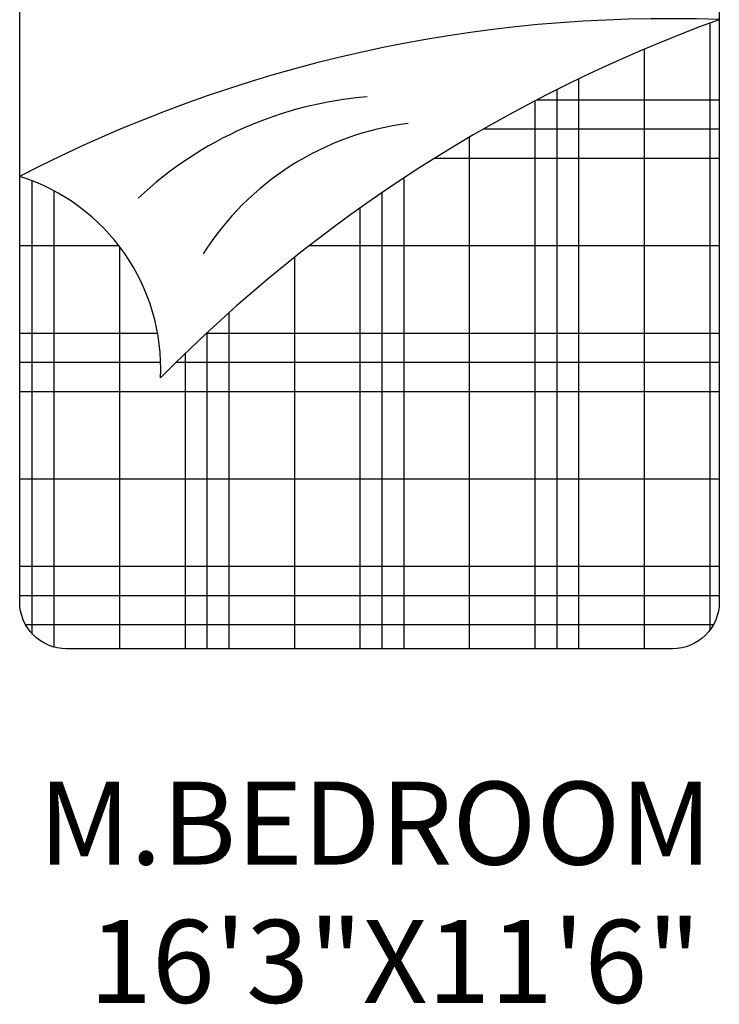
# Model space of a CAD drawing. Units: inches. Extents: x 3064 to 19385, y 846 to 15425.
# Tile 20 of 108: x 3856 to 3915, y 1289 to 1373. Entities that reach past the tile are written whole.
import ezdxf

# ---------------------------------------------------------------- set-up
doc = ezdxf.new("R2010")
doc.units = ezdxf.units.IN
doc.layers.add('A-AREA-IDEN', color=3, linetype='Continuous', lineweight=18)
doc.layers.add('A-FLOR-FIXT', color=9, linetype='Continuous', lineweight=18)
doc.layers.add('BLOCK', color=6, linetype='Continuous')
doc.styles.get("Standard").update_dxf_attribs({"font": 'arial.ttf'})

# ---------------------------------------------------------------- blocks, each defined once
blk = doc.blocks.new('*X5')
at = {"color": 0}
for p, q in [((276.598, 451.25), (280.51, 451.25)), ((275.455, 450.625), (280.51, 450.625)), ((274.411, 450), (280.51, 450)), ((265.51, 448.125), (267.634, 448.125)), ((271.723, 448.125), (280.51, 448.125)), ((265.51, 446.25), (268.465, 446.25)), ((269.519, 446.25), (280.51, 446.25)), ((265.51, 445.625), (268.531, 445.625)), ((268.866, 445.625), (280.51, 445.625)), ((265.51, 445), (280.51, 445)), ((265.51, 443.125), (280.51, 443.125)), ((265.51, 441.25), (280.51, 441.25)), ((265.51, 440.625), (280.51, 440.625)), ((265.634, 440), (280.386, 440))]:
    blk.add_line(p, q, dxfattribs=at)
blk = doc.blocks.new('*X6')
at = {"color": 0}
for p, q in [((280.312, 439.886), (280.312, 452.896)), ((278.906, 439.482), (278.906, 452.338)), ((277.5, 439.482), (277.5, 451.702)), ((277.031, 439.482), (277.031, 451.471)), ((276.562, 439.482), (276.562, 451.231)), ((275.156, 439.482), (275.156, 450.451)), ((265.781, 439.797), (265.781, 449.511)), ((273.75, 439.482), (273.75, 449.576)), ((266.25, 439.517), (266.25, 449.296)), ((273.281, 439.482), (273.281, 449.261)), ((272.812, 439.482), (272.812, 448.934)), ((267.656, 439.482), (267.656, 448.095)), ((271.406, 439.482), (271.406, 447.876)), ((270, 439.482), (270, 446.689)), ((269.531, 439.482), (269.531, 446.262)), ((269.062, 439.482), (269.062, 445.817))]:
    blk.add_line(p, q, dxfattribs=at)
blk = doc.blocks.new('A$C52E67D0D')
at = {"layer": 'BLOCK'}
blk.add_lwpolyline([(1901, 0), (601, 0, -0.414214), (501, 100), (501, 1700, -0.414214), (601, 1800), (1901, 1800, -0.414214), (2001, 1700), (2001, 100, -0.414214)], format="xyb", close=True, dxfattribs=at)
for centre, radius, start, end in [((1888.6, -1664.5), 3015.3, 87.8642, 117.4001), ((3101, -1685.8), 3227.7, 109.926, 135.3977), ((1308.8, 377.9), 807.6, 94.4436, 133.2788), ((1410.8, 520.2), 610.8, 97.2157, 147.6656), ((371.4, 600.4), 432, 357.3792, 72.5379)]:
    blk.add_arc(centre, radius, start, end, dxfattribs=at)
at = {"layer": 'BLOCK', "xscale": 100, "yscale": 100, "zscale": 100}
for name in ['*X6', '*X5']:
    blk.add_blockref(name, (-26050, -43948.2), dxfattribs=at)

msp = doc.modelspace()

# ---------------------------------------------------------------- block references
at = {"layer": 'A-FLOR-FIXT', "xscale": 0.039370099999992, "yscale": 0.039370099999992, "zscale": 0.039370099999992}
msp.add_blockref('A$C52E67D0D', (3836.607, 1319.474), dxfattribs=at)

# ---------------------------------------------------------------- texts
at = {"layer": 'A-AREA-IDEN', "insert": (3857.916, 1308.253), "char_height": 7, "attachment_point": 1}
msp.add_mtext_dynamic_manual_height_columns('M.BEDROOM\\P  16\'3"X11\'6"', width=67.59241, gutter_width=12.5, heights=[0], dxfattribs=at)

doc.saveas('drawing.dxf')
